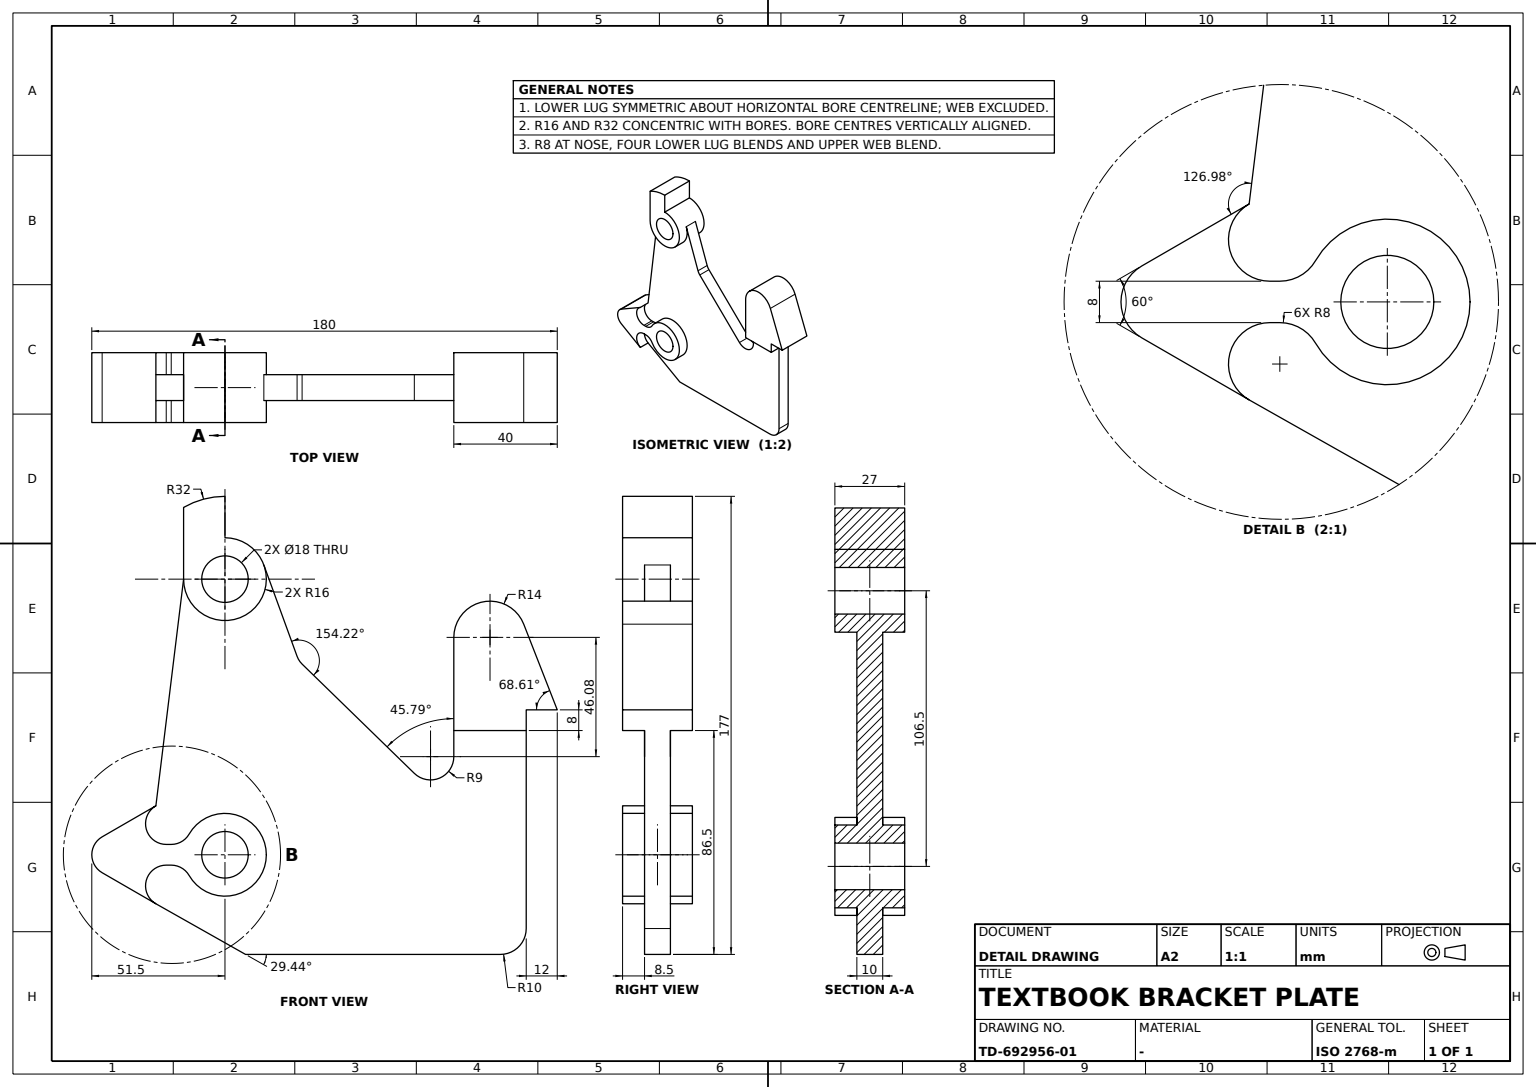
CATIA V5 part; units mm, degrees
sketch "Sketch1" plane through (0, 0, 0) normal (1, 0, 0) x (0, 1, 0)
  circle A0 centre (0, 106.5) radius 9
  point P0 (0, 106.5)
  arc A1 (-16, 106.5) -> (0, 122.5) centre (0, 106.5) ccw
  arc A2 (0, 138.5) -> (-16, 134.2128) centre (0, 106.5) ccw
  line L0 (-16, 134.2128) -> (-16, 106.5)
  line L1 (0, 122.5) -> (0, 138.5)
  dimension "radius A0" = 9
  dimension "distance P0 x axis" = 106.5
  dimension "radius A1" = 16
  dimension "radius A2" = 32
  dimension "length L1" = 16
  constraint coincidence P0 y-axis
  constraint concentricity A1 A0
  constraint concentricity A2 A1
  constraint vertical L0 y-axis
  constraint vertical L1 y-axis
  constraint tangency L0 A1
extrude "Pad1" add sketch "Sketch1" along normal mid plane 27
sketch "Sketch2" plane through (0, 0, 0) normal (1, 0, 0) x (0, 1, 0)
  circle A0 centre (0, 0) radius 9
  arc A1 (-13.8564, -8) -> (-13.8564, 8) centre (0, 0) ccw
  line L0 (-22.7154, 4) -> (-20.7846, 4)
  line L1 (-22.7154, -4) -> (-20.7846, -4)
  line L2 (0, 0) -> (-43.5, 0) construction
  line L3 (-47.5, 6.9282) -> (-26.7154, 18.9282)
  line L4 (-47.5, -6.9282) -> (-26.7154, -18.9282)
  arc A2 (-13.8564, 8) -> (-20.7846, 4) centre (-20.7846, 12) cw
  arc A3 (-26.7154, 18.9282) -> (-22.7154, 4) centre (-22.7154, 12) ccw
  point P0 (-22.7154, 12)
  arc A4 (-13.8564, -8) -> (-20.7846, -4) centre (-20.7846, -12) ccw
  arc A5 (-26.7154, -18.9282) -> (-22.7154, -4) centre (-22.7154, -12) cw
  arc A6 (-47.5, 6.9282) -> (-47.5, -6.9282) centre (-43.5, 0) ccw
  point P1 (-43.5, 0)
  dimension "radius A0" = 9
  dimension "radius A1" = 16
  dimension "distance L0 x axis" = 4
  dimension "distance L1 x axis" = 4
  dimension "angle L3 L2" = 30
  dimension "angle L4 x axis" = 30
  dimension "radius A2" = 8
  dimension "radius A3" = 8
  dimension "radius A4" = 8
  dimension "radius A5" = 8
  dimension "radius A6" = 8
  dimension "distance P1 y axis" = 43.5
  dimension "distance P0 y axis" = 22.7154
  constraint concentricity A1 A0
  constraint horizontal L0 x-axis
  constraint horizontal L1 x-axis
  constraint horizontal L2 x-axis
  constraint tangency A2 L0
  constraint tangency A2 A1
  constraint tangency A3 L3
  constraint tangency A3 L0
  constraint tangency A4 A1
  constraint tangency A4 L1
  constraint tangency A5 L4
  constraint tangency A5 L1
  constraint tangency A6 L3
  constraint tangency A6 L4
extrude "Pad2" add sketch "Sketch2" along normal mid plane 27
sketch "Sketch3" plane through (0, 0, 0) normal (1, 0, 0) x (0, 1, 0)
  line L0 (88.5, 48) -> (116.5, 48)
  line L1 (88.5, 48) -> (88.5, 84)
  point P0 (88.5, 84)
  line L2 (116.5, 48) -> (116.5, 56)
  point P1 (116.5, 56)
  line L3 (116.5, 56) -> (128.5, 56)
  arc A0 (115.5361, 89.1049) -> (88.5, 84) centre (102.5, 84) ccw
  point P2 (102.5, 84)
  line L4 (128.5, 56) -> (115.5361, 89.1049)
  dimension "length L0" = 28
  dimension "distance L0 x axis" = 48
  dimension "distance P0 x axis" = 84
  dimension "distance P1 x axis" = 56
  dimension "length L3" = 12
  dimension "distance P2 P0" = 14
  dimension "distance L2 y axis" = 116.5
  constraint horizontal L0 x-axis
  constraint horizontal L3 x-axis
  constraint vertical L1 y-axis
  constraint vertical L2 y-axis
  constraint tangency A0 L1
  constraint tangency L4 A0
extrude "Pad3" add sketch "Sketch3" along normal mid plane 27
sketch "Sketch4" plane through (0, 0, 0) normal (1, 0, 0) x (0, 1, 0)
  point P0 (79.5, 37)
  line L0 (88.5, 48) -> (116.5, 48)
  point P1 (116.5, 48)
  point P2 (28.5, 75)
  line L1 (27.8885, 76.6792) -> (15.034, 111.9752)
  arc A0 (-16, 106.5) -> (0, 122.5) centre (0, 106.5) ccw construction
  arc A1 (-16, 106.5) -> (15.034, 111.9752) centre (0, 106.5) ccw
  arc A2 (27.8885, 76.6792) -> (29.8272, 73.6825) centre (35.4055, 79.4168) ccw
  point P3 (35.4055, 79.4168)
  point P4 (15.034, 111.9752)
  point P5 (15.034, 111.9752)
  line L2 (-16, 106.5) -> (-26.7154, 18.9282)
  point P6 (-26.7154, 18.9282)
  line L3 (-26.7154, -18.9282) -> (7.9592, -38.5)
  point P7 (-26.7154, -18.9282)
  point P8 (7.9592, -38.5)
  arc A3 (-26.7154, 18.9282) -> (-22.7154, 4) centre (-22.7154, 12) ccw
  point P9 (-26.7154, 18.9282)
  arc A4 (-22.7154, -4) -> (-26.7154, -18.9282) centre (-22.7154, -12) ccw
  point P10 (-26.7154, -18.9282)
  line L4 (-20.7846, 4) -> (-22.7154, 4)
  arc A5 (-20.7846, 4) -> (-13.8564, 8) centre (-20.7846, 12) ccw
  line L5 (-22.7154, -4) -> (-20.7846, -4)
  arc A6 (-13.8564, -8) -> (-20.7846, -4) centre (-20.7846, -12) ccw
  line L6 (116.5, 48) -> (116.5, -28.5)
  line L7 (106.5, -38.5) -> (7.9592, -38.5)
  arc A7 (106.5, -38.5) -> (116.5, -28.5) centre (106.5, -28.5) ccw
  arc A8 (-13.8564, -8) -> (-13.8564, 8) centre (0, 0) ccw
  line L8 (73.2244, 31.4659) -> (29.8272, 73.6825)
  point P11 (73.2244, 31.4659)
  arc A9 (73.2244, 31.4659) -> (88.5, 37.917) centre (79.5, 37.917) ccw
  point P12 (73.2244, 31.4659)
  line L9 (88.5, 48) -> (88.5, 37.917)
  dimension "distance P0 x axis" = 37
  dimension "distance P2 x axis" = 75
  dimension "distance P2 P1 x axis" = 88
  dimension "radius A2" = 8
  dimension "distance P8 x axis" = 38.5
  dimension "angle L3 x axis" = 29.442
  dimension "radius A7" = 10
  dimension "distance P3 y axis" = 35.4055
  dimension "distance P3 x axis" = 79.4168
  dimension "distance P0 y axis" = 79.5
  dimension "length L8" = 60.5439
  dimension "radius A9" = 9
  dimension "angle L8 L9" = 45.79
  constraint tangency A0 L1
  constraint tangency A2 L1
  constraint tangency A7 L7
  constraint tangency A7 L6
  constraint tangency L8 A2
  constraint tangency A9 L8
  constraint coincidence L1 P4
  constraint coincidence A0 P5
  constraint coincidence P7 P10
  constraint coincidence P6 P9
  constraint coincidence L8 P12
  constraint coincidence P12 P11
  constraint coincidence P4 P5
  constraint vertical L6 y-axis
  constraint vertical L9 y-axis
  constraint horizontal L7 x-axis
extrude "Pad4" add sketch "Sketch4" along normal mid plane 10
